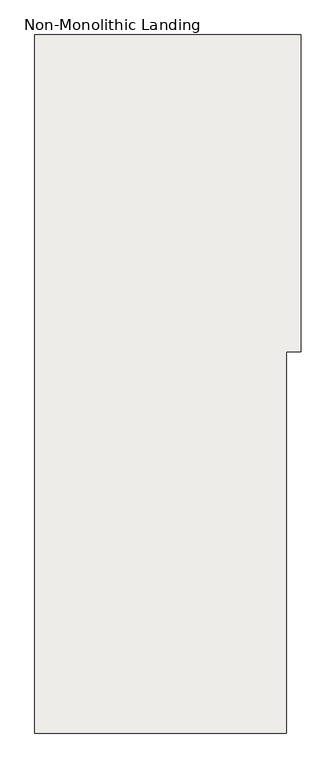
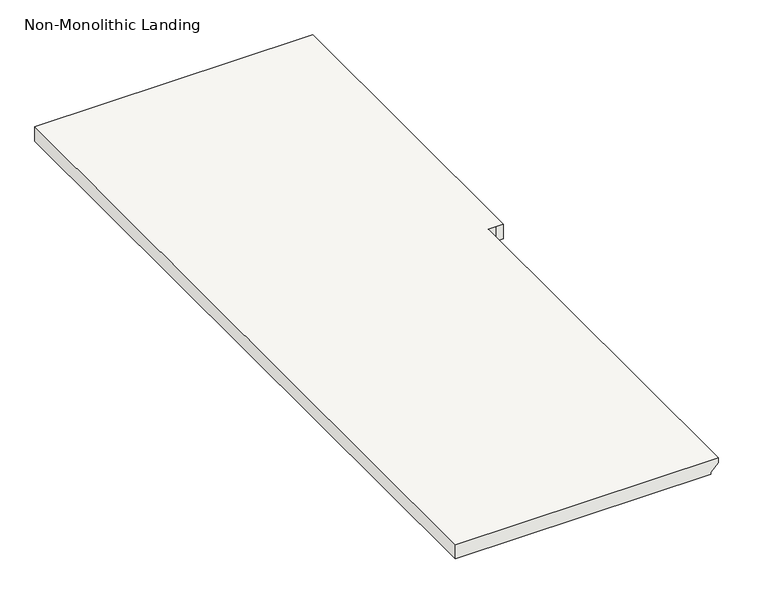
"""IFC4 building model written with IfcOpenShell, lengths in millimetres: slab geometry, Non-Monolithic Landing."""

from ifc_helpers import new_model, si_unit, origin, place, context, project, spatial, faceted_brep, source, transform, mapped, element, save


def non_monolithic_landing_077bd761(model_context):
    return source(origin(), model_context, "Body", "Brep", [
        faceted_brep([(-10221.4683044, -3838.3891189, 4781.55), (-10246.8683044, -3838.3891189, 4756.15), (-10246.8683044, -2706.1923176, 4756.15), (-10221.4683044, -2706.1923176, 4781.55), (-10221.4683044, -2492.1891189, 4800.6), (-10196.0683044, -2492.1891189, 4800.6), (-10170.6683044, -2492.1891189, 4800.6), (-10170.6683044, -1374.5891189, 4800.6), (-10196.0683044, -1374.5891189, 4800.6), (-11110.4683044, -1374.5891189, 4800.6), (-11110.4683044, -3838.3891189, 4800.6), (-10221.4683044, -3838.3891189, 4800.6), (-10246.8683044, -2706.1923176, 4749.8), (-10246.8683044, -3838.3891189, 4749.8), (-11110.4683044, -3838.3891189, 4749.8), (-11110.4683044, -1374.5891189, 4749.8), (-10196.0683044, -1374.5891189, 4749.8), (-10170.6683044, -1374.5891189, 4749.8), (-10170.6683044, -2492.1891189, 4749.8), (-10196.0683044, -2492.1891189, 4749.8), (-10221.4683044, -2492.1891189, 4749.8), (-10221.4683044, -2706.1923176, 4749.8)], [[[0, 1, 2, 3]], [[4, 5, 6, 7, 8, 9, 10, 11]], [[12, 13, 14, 15, 16, 17, 18, 19, 20, 21]], [[13, 12, 2, 1]], [[12, 21, 3, 2]], [[4, 11, 0, 3, 21, 20]], [[9, 8, 16, 15]], [[10, 9, 15, 14]], [[11, 10, 14, 13, 1, 0]], [[5, 4, 20, 19]], [[6, 5, 19, 18]], [[7, 6, 18, 17]], [[8, 7, 17, 16]]]),
    ])


if __name__ == "__main__":
    model = new_model("IFC4")
    model_context = context("Model", 3, world=origin())
    ifc_project = project(units=[si_unit("LENGTHUNIT", "METRE", prefix="MILLI")], contexts=[model_context])
    site = spatial("IfcSite", under=ifc_project)
    building = spatial("IfcBuilding", under=site)
    placement = place(None, origin())
    non_monolithic_landing_shape = non_monolithic_landing_077bd761(model_context)
    element("IfcSlab", 1, ObjectType="Non-Monolithic Landing", at=placement, inside=building, context=model_context, shape_type="MappedRepresentation", body=[
        mapped(non_monolithic_landing_shape, transform((0.0, 0.0, 0.0), x_axis=(1.0, 0.0, 0.0), y_axis=(0.0, 1.0, 0.0), z_axis=(0.0, 0.0, 1.0))),
    ])
    save(model, "model.ifc")
